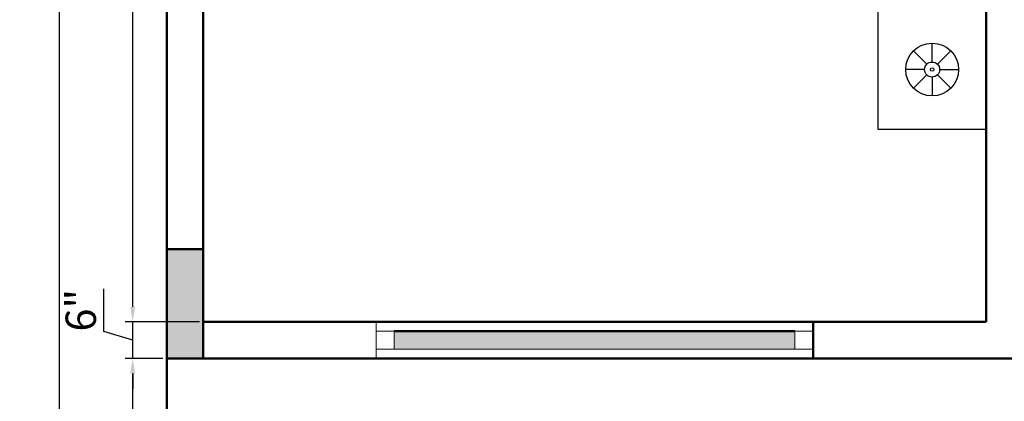
# Model space of a CAD drawing. Units: inches. Extents: x 3064 to 19385, y 846 to 15425.
# Tile 66 of 108: x 6445 to 6607, y 1561 to 1624. Entities that reach past the tile are written whole.
import ezdxf

# ---------------------------------------------------------------- set-up
doc = ezdxf.new("R2010")
doc.units = ezdxf.units.IN
for name, color, linetype, lineweight in [('A-ANNO-DIMS', 2, 'Continuous', 18), ('A-COLS', 1, 'Continuous', 35), ('A-FLOR-FIXT', 9, 'Continuous', 18), ('A-GLAZ', 4, 'Continuous', 18), ('A-WALL', 7, 'Continuous', 50)]:
    doc.layers.add(name, color=color, linetype=linetype, lineweight=lineweight)
doc.layers.add('BLOCK', color=6, linetype='Continuous')
doc.styles.get("Standard").update_dxf_attribs({"font": 'arial.ttf'})
doc.dimstyles.new('ISO-25', dxfattribs={"dimtxt": 9, "dimasz": 2.5, "dimexe": 1.25, "dimexo": 0.625, "dimtad": 1, "dimdec": 1, "dimlunit": 3, "dimtxsty": 'Standard', "dimcen": 2.5, "dimadec": 0, "dimazin": 0, "dimtfac": 1, "dimtdec": 1, "dimtmove": 0, "dimatfit": 3, "dimfxl": 1, "dimarcsym": 0})

# ---------------------------------------------------------------- blocks, each defined once
blk = doc.blocks.new('A$C52E67D0D')
at = {"layer": 'BLOCK'}
for p, q in [((2229.3, 1596.3), (2173.3, 1652.3)), ((2251.5, 1605.5), (2251.5, 1684.7)), ((2273.7, 1596.3), (2329.7, 1652.3)), ((2220.1, 1574.1), (2140.9, 1574.1)), ((2282.9, 1574.1), (2362.1, 1574.1)), ((2229.3, 1551.9), (2173.3, 1495.9)), ((2251.5, 1542.8), (2251.5, 1463.5)), ((2273.7, 1551.9), (2329.7, 1495.9))]:
    blk.add_line(p, q, dxfattribs=at)
blk.add_lwpolyline([(2001, 1348.6), (2001, 1799.6), (2502, 1799.6), (2502, 1348.6)], close=True, dxfattribs=at)
for radius in [110.6, 31.4, 7.46]:
    blk.add_circle((2251.5, 1574.1), radius, dxfattribs=at)
blk = doc.blocks.new('*D379')
at = {"layer": 'A-ANNO-DIMS', "color": 0, "lineweight": -2, "transparency": 16777216}
for p, q in [((6468.41, 1567.99), (6462.18, 1567.99)), ((6463.43, 1498.49), (6463.43, 1565.49)), ((6468.41, 1495.99), (6462.18, 1495.99))]:
    blk.add_line(p, q, dxfattribs=at)
at = {"layer": 'A-ANNO-DIMS', "color": 0, "transparency": 16777216}
for points in [[(6463.02, 1565.49), (6463.85, 1565.49), (6463.43, 1567.99)], [(6463.02, 1498.49), (6463.85, 1498.49), (6463.43, 1495.99)]]:
    blk.add_solid(points, dxfattribs=at)
at = {"layer": 'Defpoints', "color": 0, "transparency": 16777216}
for p in [(6463.43, 1567.99), (6469.03, 1567.99), (6469.03, 1495.99)]:
    blk.add_point(p, dxfattribs=at)
at = {"layer": 'A-ANNO-DIMS', "color": 0, "transparency": 16777216, "insert": (6460.26, 1531.99), "char_height": 5, "attachment_point": 5, "rotation": 90}
blk.add_mtext("6'", dxfattribs=at)
blk = doc.blocks.new('*D371')
at = {"layer": 'A-ANNO-DIMS', "color": 0, "lineweight": -2, "transparency": 16777216}
for p, q in [((6458.69, 1572.41), (6458.69, 1579.44)), ((6463.43, 1576.49), (6463.43, 1578.99)), ((6474.41, 1573.99), (6462.18, 1573.99)), ((6463.43, 1567.99), (6463.43, 1573.99)), ((6463.43, 1567.99), (6463.43, 1573.99)), ((6463.43, 1570.99), (6458.69, 1572.41)), ((6468.41, 1567.99), (6462.18, 1567.99)), ((6463.43, 1565.49), (6463.43, 1562.99))]:
    blk.add_line(p, q, dxfattribs=at)
at = {"layer": 'A-ANNO-DIMS', "color": 0, "transparency": 16777216}
for points in [[(6463.02, 1576.49), (6463.85, 1576.49), (6463.43, 1573.99)], [(6463.02, 1565.49), (6463.85, 1565.49), (6463.43, 1567.99)]]:
    blk.add_solid(points, dxfattribs=at)
at = {"layer": 'Defpoints', "color": 0, "transparency": 16777216}
for p in [(6463.43, 1573.99), (6475.03, 1573.99), (6469.03, 1567.99)]:
    blk.add_point(p, dxfattribs=at)
at = {"layer": 'A-ANNO-DIMS', "color": 0, "transparency": 16777216, "insert": (6455.52, 1575.92), "char_height": 5, "attachment_point": 5, "rotation": 90}
blk.add_mtext('6"', dxfattribs=at)
blk = doc.blocks.new('*D372')
at = {"layer": 'A-ANNO-DIMS', "color": 0, "lineweight": -2, "transparency": 16777216}
for p, q in [((6474.41, 1771.99), (6462.18, 1771.99)), ((6463.43, 1576.49), (6463.43, 1769.49)), ((6474.41, 1573.99), (6462.18, 1573.99))]:
    blk.add_line(p, q, dxfattribs=at)
at = {"layer": 'A-ANNO-DIMS', "color": 0, "transparency": 16777216}
for points in [[(6463.02, 1769.49), (6463.85, 1769.49), (6463.43, 1771.99)], [(6463.02, 1576.49), (6463.85, 1576.49), (6463.43, 1573.99)]]:
    blk.add_solid(points, dxfattribs=at)
at = {"layer": 'Defpoints', "color": 0, "transparency": 16777216}
for p in [(6463.43, 1771.99), (6475.03, 1771.99), (6475.03, 1573.99)]:
    blk.add_point(p, dxfattribs=at)
at = {"layer": 'A-ANNO-DIMS', "color": 0, "transparency": 16777216, "insert": (6460.26, 1672.99), "char_height": 5, "attachment_point": 5, "rotation": 90}
blk.add_mtext('16\'-6"', dxfattribs=at)
blk = doc.blocks.new('*D370')
at = {"layer": 'A-ANNO-DIMS', "color": 0, "lineweight": -2, "transparency": 16777216}
for p, q in [((6468.41, 1987.99), (6450.1, 1987.99)), ((6451.35, 1498.49), (6451.35, 1985.49)), ((6468.41, 1495.99), (6450.1, 1495.99))]:
    blk.add_line(p, q, dxfattribs=at)
at = {"layer": 'A-ANNO-DIMS', "color": 0, "transparency": 16777216}
for points in [[(6450.94, 1985.49), (6451.77, 1985.49), (6451.35, 1987.99)], [(6450.94, 1498.49), (6451.77, 1498.49), (6451.35, 1495.99)]]:
    blk.add_solid(points, dxfattribs=at)
at = {"layer": 'Defpoints', "color": 0, "transparency": 16777216}
for p in [(6451.35, 1987.99), (6469.03, 1987.99), (6469.03, 1495.99)]:
    blk.add_point(p, dxfattribs=at)
at = {"layer": 'A-ANNO-DIMS', "color": 0, "transparency": 16777216, "insert": (6448.22, 1741.99), "char_height": 5, "attachment_point": 5, "rotation": 90}
blk.add_mtext("41'", dxfattribs=at)
blk = doc.blocks.new('WIN-1900')
blk.add_line((3, 0), (3, 66))
blk.add_lwpolyline([(3, 66), (0, 66), (0, 69), (3, 69)], close=True)

msp = doc.modelspace()

# ---------------------------------------------------------------- hatches: boundary and pattern name
at = {"layer": 'A-COLS'}
h = msp.add_hatch(color=256, dxfattribs=at)
h.dxf.hatch_style = 1
h.paths.add_polyline_path([(6469.03, 1567.99), (6475.03, 1567.99), (6475.03, 1585.99), (6469.03, 1585.99)])
at = {"layer": 'A-GLAZ'}
h = msp.add_hatch(color=256, dxfattribs=at)
h.dxf.hatch_style = 1
h.paths.add_polyline_path([(6506.53, 1572.49), (6506.53, 1569.49), (6572.53, 1569.49), (6572.53, 1572.49)])

# ---------------------------------------------------------------- linework, layer by layer
msp.add_line((6503.53, 1567.99), (6503.53, 1573.99), dxfattribs=at)
msp.add_lwpolyline([(6503.53, 1569.49), (6503.53, 1572.49), (6506.53, 1572.49), (6506.53, 1569.49)], close=True, dxfattribs=at)
at = {"layer": 'A-WALL'}
for p, q in [((6469.03, 1987.99), (6469.03, 1567.99)), ((6475.03, 1771.99), (6475.03, 1573.99)), ((6604.03, 1735.99), (6604.03, 1573.99)), ((6604.03, 1573.99), (6475.03, 1573.99)), ((6575.53, 1567.99), (6575.53, 1573.99)), ((6506.53, 1572.49), (6572.53, 1572.49)), ((6811.03, 1567.99), (6469.03, 1567.99)), ((6475.03, 1567.99), (6469.03, 1567.99)), ((6469.03, 1567.99), (6469.03, 1495.99))]:
    msp.add_line(p, q, dxfattribs=at)
msp.add_lwpolyline([(6475.03, 1567.99), (6475.03, 1585.99), (6469.03, 1585.99), (6469.03, 1567.99)], close=True, dxfattribs=at)

# ---------------------------------------------------------------- block references
at = {"layer": 'A-FLOR-FIXT', "xscale": 0.039370099999992, "yscale": 0.039370099999992, "zscale": 0.039370099999992, "rotation": 270}
msp.add_blockref('A$C52E67D0D', (6533.17, 1704.24), dxfattribs=at)
at = {"layer": 'A-GLAZ', "rotation": 269.9999999999993}
msp.add_blockref('WIN-1900', (6506.53, 1572.49), dxfattribs=at)

# ---------------------------------------------------------------- dimensions: what is measured, and where the dimension line sits
at = {"layer": 'A-ANNO-DIMS'}
for base, p1, p2, override, picture, middle in [((6451.35, 1987.99), (6469.03, 1495.99), (6469.03, 1987.99), {"dimtxt": 5, "dimclrd": 0, "dimclre": 0, "dimclrt": 0}, '*D370', (6448.22, 1741.99)), ((6463.43, 1771.99), (6475.03, 1573.99), (6475.03, 1771.99), {"dimtxt": 5, "dimclrd": 0, "dimclre": 0, "dimclrt": 0, "dimtmove": 1}, '*D372', (6460.26, 1672.99)), ((6463.43, 1573.99), (6469.03, 1567.99), (6475.03, 1573.99), {"dimtxt": 5, "dimclrd": 0, "dimclre": 0, "dimclrt": 0, "dimtmove": 1}, '*D371', (6455.52, 1573.04)), ((6463.43, 1567.99), (6469.03, 1495.99), (6469.03, 1567.99), {"dimtxt": 5, "dimclrd": 0, "dimclre": 0, "dimclrt": 0}, '*D379', (6460.26, 1531.99))]:
    dim = msp.add_linear_dim(base=base, p1=p1, p2=p2, angle=90, dimstyle='ISO-25', override=override, dxfattribs=at)
    dim.commit()
    dim.dimension.update_dxf_attribs({"geometry": picture, "text_midpoint": middle})

doc.saveas('drawing.dxf')
